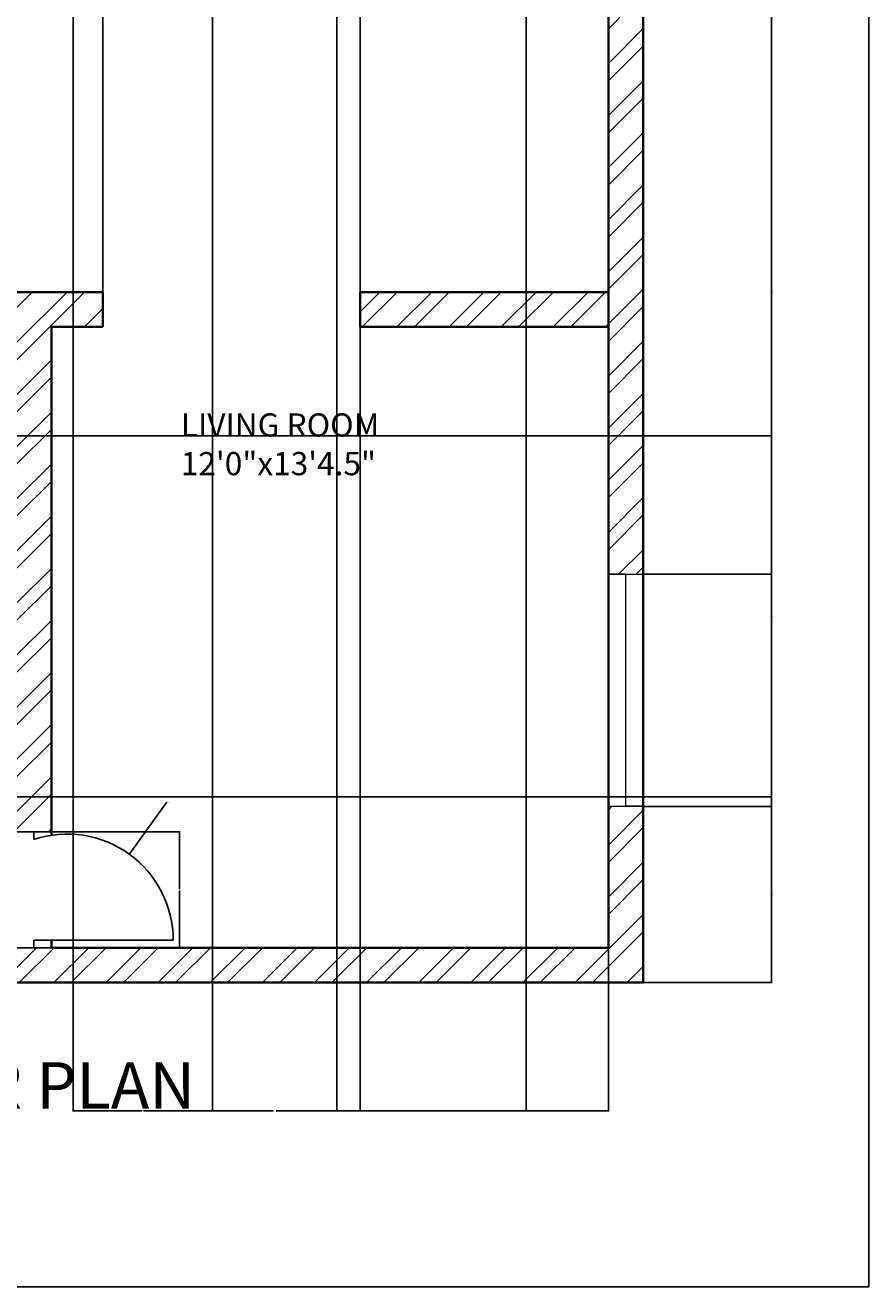
# Model space of a CAD drawing. Units: inches. Extents: x 1595 to 2135, y 460 to 2061.
# Tile 3 of 5: x 1917 to 2135, y 1320 to 1646. Entities that reach past the tile are written whole.
import ezdxf

# ---------------------------------------------------------------- set-up
doc = ezdxf.new("R2010")
doc.units = ezdxf.units.IN
for name, color, linetype, lineweight in [('A-ANNO-DIMS', 2, 'Continuous', 18), ('A-ANNO-TTLB', 7, 'Continuous', 25), ('A-AREA-IDEN', 7, 'Continuous', 18), ('A-DOOR', 3, 'Continuous', 25), ('A-GLAZ', 4, 'Continuous', 18), ('A-WALL', 7, 'Continuous', 35)]:
    doc.layers.add(name, color=color, linetype=linetype, lineweight=lineweight)
doc.layers.add('A-WALL-PATT', color=143, linetype='Continuous', lineweight=13, true_color=0x7aafdf)
doc.styles.get("Standard").update_dxf_attribs({"font": 'arial.ttf'})
doc.dimstyles.get("Standard").update_dxf_attribs({"dimtxt": 0.18, "dimasz": 0.18, "dimexe": 0.18, "dimexo": 0.0625, "dimgap": 0.09, "dimtad": 0, "dimtih": 1, "dimtoh": 1, "dimdec": 4, "dimzin": 0, "dimdsep": 46, "dimtxsty": 'Standard', "dimcen": 0.09, "dimadec": 0, "dimazin": 0, "dimtfac": 1, "dimtdec": 4, "dimtofl": 0, "dimtmove": 0, "dimatfit": 3, "dimfxl": 1, "dimtolj": 1, "dimtzin": 0, "dimarcsym": 0})

# ---------------------------------------------------------------- blocks, each defined once
blk = doc.blocks.new('WIN-60IN')
for p, q in [((4.5, 60), (0, 60)), ((0, 60), (9, 60)), ((4.5, 0), (4.5, 60)), ((0, 0), (9, 0)), ((9, 0), (4.5, 0))]:
    blk.add_line(p, q)
blk = doc.blocks.new('*D14')
at = {"layer": 'A-ANNO-DIMS', "color": 0, "lineweight": -2, "transparency": 16777216}
for p, q in [((2076.38, 1444.2), (2109.64, 1444.2)), ((2109.46, 1444.02), (2109.46, 1421.6)), ((2109.46, 1398.82), (2109.46, 1421.24)), ((2076.38, 1398.64), (2109.64, 1398.64))]:
    blk.add_line(p, q, dxfattribs=at)
at = {"layer": 'A-ANNO-DIMS', "color": 0, "transparency": 16777216}
for points in [[(2109.43, 1444.02), (2109.49, 1444.02), (2109.46, 1444.2)], [(2109.43, 1398.82), (2109.49, 1398.82), (2109.46, 1398.64)]]:
    blk.add_solid(points, dxfattribs=at)
at = {"layer": 'Defpoints', "color": 0, "transparency": 16777216}
for p in [(2076.31, 1444.2), (2109.46, 1444.2), (2076.31, 1398.64)]:
    blk.add_point(p, dxfattribs=at)
at = {"layer": 'A-ANNO-DIMS', "color": 0, "transparency": 16777216, "insert": (2109.46, 1421.42), "char_height": 0.18, "attachment_point": 5}
blk.add_mtext('\\A1;45.56', dxfattribs=at)
blk = doc.blocks.new('*D15')
at = {"layer": 'A-ANNO-DIMS', "color": 0, "lineweight": -2, "transparency": 16777216}
for p, q in [((2076.38, 1650.64), (2109.64, 1650.64)), ((2109.46, 1650.46), (2109.46, 1577.6)), ((2109.46, 1504.38), (2109.46, 1577.24)), ((2076.38, 1504.2), (2109.64, 1504.2))]:
    blk.add_line(p, q, dxfattribs=at)
at = {"layer": 'A-ANNO-DIMS', "color": 0, "transparency": 16777216}
for points in [[(2109.43, 1650.46), (2109.49, 1650.46), (2109.46, 1650.64)], [(2109.43, 1504.38), (2109.49, 1504.38), (2109.46, 1504.2)]]:
    blk.add_solid(points, dxfattribs=at)
at = {"layer": 'Defpoints', "color": 0, "transparency": 16777216}
for p in [(2076.31, 1650.64), (2109.46, 1650.64), (2076.31, 1504.2)]:
    blk.add_point(p, dxfattribs=at)
at = {"layer": 'A-ANNO-DIMS', "color": 0, "transparency": 16777216, "insert": (2109.46, 1577.42), "char_height": 0.18, "attachment_point": 5}
blk.add_mtext('\\A1;146.44', dxfattribs=at)
blk = doc.blocks.new('*D20')
at = {"layer": 'A-ANNO-DIMS', "color": 0, "lineweight": -2, "transparency": 16777216}
for p, q in [((1923.38, 1437.64), (1956.64, 1437.64)), ((1956.46, 1437.46), (1956.46, 1422.82)), ((1956.46, 1407.82), (1956.46, 1422.46)), ((1923.38, 1407.64), (1956.64, 1407.64))]:
    blk.add_line(p, q, dxfattribs=at)
at = {"layer": 'A-ANNO-DIMS', "color": 0, "transparency": 16777216}
for points in [[(1956.43, 1437.46), (1956.49, 1437.46), (1956.46, 1437.64)], [(1956.43, 1407.82), (1956.49, 1407.82), (1956.46, 1407.64)]]:
    blk.add_solid(points, dxfattribs=at)
at = {"layer": 'Defpoints', "color": 0, "transparency": 16777216}
for p in [(1923.31, 1437.64), (1923.31, 1407.64), (1956.46, 1407.64)]:
    blk.add_point(p, dxfattribs=at)
at = {"layer": 'A-ANNO-DIMS', "color": 0, "transparency": 16777216, "insert": (1956.46, 1422.64), "char_height": 0.18, "attachment_point": 5}
blk.add_mtext('\\A1;30', dxfattribs=at)
blk = doc.blocks.new('*D21')
at = {"layer": 'A-ANNO-DIMS', "color": 0, "lineweight": -2, "transparency": 16777216}
for p, q in [((1936.61, 1577.2), (1936.61, 2049.97)), ((1936.79, 2049.79), (1969.47, 2049.79)), ((2002.95, 2049.79), (1970.26, 2049.79)), ((2003.13, 1577.2), (2003.13, 2049.97))]:
    blk.add_line(p, q, dxfattribs=at)
at = {"layer": 'A-ANNO-DIMS', "color": 0, "transparency": 16777216}
for points in [[(1936.79, 2049.82), (1936.79, 2049.76), (1936.61, 2049.79)], [(2002.95, 2049.82), (2002.95, 2049.76), (2003.13, 2049.79)]]:
    blk.add_solid(points, dxfattribs=at)
at = {"layer": 'Defpoints', "color": 0, "transparency": 16777216}
for p in [(2003.13, 2049.79), (1936.61, 1577.14), (2003.13, 1577.14)]:
    blk.add_point(p, dxfattribs=at)
at = {"layer": 'A-ANNO-DIMS', "color": 0, "transparency": 16777216, "insert": (1969.87, 2049.79), "char_height": 0.18, "attachment_point": 5}
blk.add_mtext('\\A1;66.52', dxfattribs=at)
blk = doc.blocks.new('*D22')
at = {"layer": 'A-ANNO-DIMS', "color": 0, "lineweight": -2, "transparency": 16777216}
for p, q in [((2003.13, 1568.08), (2003.13, 1365.31)), ((2067.31, 1568.08), (2067.31, 1365.31)), ((2003.31, 1365.49), (2034.83, 1365.49)), ((2067.13, 1365.49), (2035.62, 1365.49))]:
    blk.add_line(p, q, dxfattribs=at)
at = {"layer": 'A-ANNO-DIMS', "color": 0, "transparency": 16777216}
for points in [[(2003.31, 1365.52), (2003.31, 1365.46), (2003.13, 1365.49)], [(2067.13, 1365.52), (2067.13, 1365.46), (2067.31, 1365.49)]]:
    blk.add_solid(points, dxfattribs=at)
at = {"layer": 'Defpoints', "color": 0, "transparency": 16777216}
for p in [(2003.13, 1568.14), (2067.31, 1568.14), (2067.31, 1365.49)]:
    blk.add_point(p, dxfattribs=at)
at = {"layer": 'A-ANNO-DIMS', "color": 0, "transparency": 16777216, "insert": (2035.22, 1365.49), "char_height": 0.18, "attachment_point": 5}
blk.add_mtext('\\A1;64.18', dxfattribs=at)
blk = doc.blocks.new('*D27')
at = {"layer": 'A-ANNO-DIMS', "color": 0, "lineweight": -2, "transparency": 16777216}
for p, q in [((1997.11, 1938.58), (1997.11, 1365.31)), ((2046.03, 1938.58), (2046.03, 1365.31)), ((1997.29, 1365.49), (2021.18, 1365.49)), ((2045.85, 1365.49), (2021.97, 1365.49))]:
    blk.add_line(p, q, dxfattribs=at)
at = {"layer": 'A-ANNO-DIMS', "color": 0, "transparency": 16777216}
for points in [[(1997.29, 1365.52), (1997.29, 1365.46), (1997.11, 1365.49)], [(2045.85, 1365.52), (2045.85, 1365.46), (2046.03, 1365.49)]]:
    blk.add_solid(points, dxfattribs=at)
at = {"layer": 'Defpoints', "color": 0, "transparency": 16777216}
for p in [(1997.11, 1938.64), (2046.03, 1938.64), (2046.03, 1365.49)]:
    blk.add_point(p, dxfattribs=at)
at = {"layer": 'A-ANNO-DIMS', "color": 0, "transparency": 16777216, "insert": (2021.57, 1365.49), "char_height": 0.18, "attachment_point": 5}
blk.add_mtext('\\A1;48.92', dxfattribs=at)
blk = doc.blocks.new('*D28')
at = {"layer": 'A-ANNO-DIMS', "color": 0, "lineweight": -2, "transparency": 16777216}
for p, q in [((1928.93, 1938.58), (1928.93, 1365.31)), ((1964.93, 1938.58), (1964.93, 1365.31)), ((1929.11, 1365.49), (1946.71, 1365.49)), ((1964.75, 1365.49), (1947.15, 1365.49))]:
    blk.add_line(p, q, dxfattribs=at)
at = {"layer": 'A-ANNO-DIMS', "color": 0, "transparency": 16777216}
for points in [[(1929.11, 1365.52), (1929.11, 1365.46), (1928.93, 1365.49)], [(1964.75, 1365.52), (1964.75, 1365.46), (1964.93, 1365.49)]]:
    blk.add_solid(points, dxfattribs=at)
at = {"layer": 'Defpoints', "color": 0, "transparency": 16777216}
for p in [(1928.93, 1938.64), (1964.93, 1938.64), (1964.93, 1365.49)]:
    blk.add_point(p, dxfattribs=at)
at = {"layer": 'A-ANNO-DIMS', "color": 0, "transparency": 16777216, "insert": (1946.93, 1365.49), "char_height": 0.18, "attachment_point": 5}
blk.add_mtext('\\A1;36', dxfattribs=at)
blk = doc.blocks.new('*D29')
at = {"layer": 'A-ANNO-DIMS', "color": 0, "lineweight": -2, "transparency": 16777216}
for p, q in [((1964.93, 1938.58), (1964.93, 1365.31)), ((1997.11, 1938.58), (1997.11, 1365.31)), ((1965.11, 1365.49), (1980.63, 1365.49)), ((1996.93, 1365.49), (1981.42, 1365.49))]:
    blk.add_line(p, q, dxfattribs=at)
at = {"layer": 'A-ANNO-DIMS', "color": 0, "transparency": 16777216}
for points in [[(1965.11, 1365.52), (1965.11, 1365.46), (1964.93, 1365.49)], [(1996.93, 1365.52), (1996.93, 1365.46), (1997.11, 1365.49)]]:
    blk.add_solid(points, dxfattribs=at)
at = {"layer": 'Defpoints', "color": 0, "transparency": 16777216}
for p in [(1964.93, 1938.64), (1997.11, 1938.64), (1997.11, 1365.49)]:
    blk.add_point(p, dxfattribs=at)
at = {"layer": 'A-ANNO-DIMS', "color": 0, "transparency": 16777216, "insert": (1981.02, 1365.49), "char_height": 0.18, "attachment_point": 5}
blk.add_mtext('\\A1;32.18', dxfattribs=at)
blk = doc.blocks.new('*D34')
at = {"layer": 'A-ANNO-DIMS', "color": 0, "lineweight": -2, "transparency": 16777216}
for p, q in [((1914.38, 1539.98), (2109.64, 1539.98)), ((2109.46, 1539.8), (2109.46, 1493.49)), ((2109.46, 1446.82), (2109.46, 1493.13)), ((1914.38, 1446.64), (2109.64, 1446.64))]:
    blk.add_line(p, q, dxfattribs=at)
at = {"layer": 'A-ANNO-DIMS', "color": 0, "transparency": 16777216}
for points in [[(2109.43, 1539.8), (2109.49, 1539.8), (2109.46, 1539.98)], [(2109.43, 1446.82), (2109.49, 1446.82), (2109.46, 1446.64)]]:
    blk.add_solid(points, dxfattribs=at)
at = {"layer": 'Defpoints', "color": 0, "transparency": 16777216}
for p in [(1914.31, 1539.98), (2109.46, 1539.98), (1914.31, 1446.64)]:
    blk.add_point(p, dxfattribs=at)
at = {"layer": 'A-ANNO-DIMS', "color": 0, "transparency": 16777216, "insert": (2109.46, 1493.31), "char_height": 0.18, "attachment_point": 5}
blk.add_mtext('\\A1;93.33', dxfattribs=at)
blk = doc.blocks.new('*D46')
at = {"layer": 'A-ANNO-DIMS', "color": 0, "lineweight": -2, "transparency": 16777216}
for p, q in [((2076.38, 2016.64), (2109.64, 2016.64)), ((2109.46, 2016.46), (2109.46, 1707.82)), ((2109.46, 1398.82), (2109.46, 1707.46)), ((2076.38, 1398.64), (2109.64, 1398.64))]:
    blk.add_line(p, q, dxfattribs=at)
at = {"layer": 'A-ANNO-DIMS', "color": 0, "transparency": 16777216}
for points in [[(2109.43, 2016.46), (2109.49, 2016.46), (2109.46, 2016.64)], [(2109.43, 1398.82), (2109.49, 1398.82), (2109.46, 1398.64)]]:
    blk.add_solid(points, dxfattribs=at)
at = {"layer": 'Defpoints', "color": 0, "transparency": 16777216}
for p in [(2076.31, 2016.64), (2109.46, 2016.64), (2076.31, 1398.64)]:
    blk.add_point(p, dxfattribs=at)
at = {"layer": 'A-ANNO-DIMS', "color": 0, "transparency": 16777216, "insert": (2109.46, 1707.64), "char_height": 0.18, "attachment_point": 5}
blk.add_mtext('\\A1;618', dxfattribs=at)
blk = doc.blocks.new('*D59')
at = {"layer": 'A-ANNO-DIMS', "color": 0, "lineweight": -2, "transparency": 16777216}
for p, q in [((1953.08, 1445.17), (1943.57, 1431.99)), ((1953.26, 1445.17), (1953.08, 1445.17)), ((1927.33, 1409.64), (1927.51, 1409.64)), ((1927.42, 1409.55), (1927.42, 1409.73))]:
    blk.add_line(p, q, dxfattribs=at)
at = {"layer": 'A-ANNO-DIMS', "color": 0, "transparency": 16777216}
blk.add_solid([(1943.54, 1432.01), (1943.59, 1431.97), (1943.46, 1431.85)], dxfattribs=at)
at = {"layer": 'Defpoints', "color": 0, "transparency": 16777216}
for p in [(1943.46, 1431.85), (1927.42, 1409.64)]:
    blk.add_point(p, dxfattribs=at)
at = {"layer": 'A-ANNO-DIMS', "color": 0, "transparency": 16777216, "insert": (1953.74, 1445.17), "char_height": 0.18, "attachment_point": 5}
blk.add_mtext('\\A1;R27.39', dxfattribs=at)

msp = doc.modelspace()

# ---------------------------------------------------------------- hatches: boundary and pattern name
at = {"layer": 'A-WALL-PATT'}
h = msp.add_hatch(dxfattribs=at)
h.set_pattern_fill('ANSI32', color=256)
h.paths.add_polyline_path([(2076.313, 2016.6421), (1674.313, 2016.6421), (1674.313, 1905.0731), (1683.313, 1905.0731), (1683.313, 1938.6421), (1705.9756, 1938.6421), (1705.9756, 1947.6421), (1683.313, 1947.6421), (1683.313, 2007.6421), (2067.313, 2007.6421), (2067.313, 1947.6421), (2046.0304, 1947.6421), (2046.0304, 1938.6421), (2067.313, 1938.6421), (2067.313, 1906.0373), (2076.313, 1906.0373), (2076.313, 1947.6421)])
h.paths.add_polyline_path([(1786.653, 1947.6421), (1748.8699, 1947.6421), (1748.8699, 1938.6421), (1786.653, 1938.6421), (1786.653, 1943.1421)], flags=17)
h.paths.add_polyline_path([(1843.367, 1943.1421), (1843.367, 1947.6421), (1822.653, 1947.6421), (1822.653, 1938.6421), (1827.313, 1938.6421), (1827.313, 1821.1082), (1836.313, 1821.1082), (1836.313, 1938.6421), (1843.367, 1938.6421)])
h.paths.add_polyline_path([(1928.933, 1943.1421), (1928.933, 1947.6421), (1875.313, 1947.6421), (1875.313, 1938.6421), (1914.313, 1938.6421), (1914.313, 1820.8892), (1923.313, 1820.8892), (1923.313, 1938.6421), (1928.933, 1938.6421)])
h.paths.add_polyline_path([(1997.1133, 1947.6421), (1964.933, 1947.6421), (1964.933, 1938.6421), (1997.1133, 1938.6421)], flags=17)
h.paths.add_polyline_path([(1974.313, 2007.6421), (1969.813, 2007.6421), (1969.813, 1947.6421), (1974.313, 1947.6421)], flags=17)
h.paths.add_polyline_path([(1780.813, 2007.6421), (1776.313, 2007.6421), (1776.313, 1947.6421), (1780.813, 1947.6421)], flags=17)
h.paths.add_polyline_path([(1683.313, 1845.0731), (1674.313, 1845.0731), (1674.313, 1734.209), (1683.313, 1734.209), (1683.313, 1773.6421), (1795.813, 1773.6421), (1836.313, 1773.6421), (1836.313, 1788.3627), (1831.813, 1788.3627), (1827.313, 1788.3627), (1827.313, 1782.6421), (1683.313, 1782.6421)])
h.paths.add_polyline_path([(2076.313, 1846.0373), (2067.313, 1846.0373), (2067.313, 1782.6421), (1923.313, 1782.6421), (1923.313, 1788.8802), (1918.813, 1788.8802), (1914.313, 1788.8802), (1914.313, 1773.6421), (2067.313, 1773.6421), (2067.313, 1710.6421), (2076.313, 1710.6421)])
h.paths.add_polyline_path([(1844.0531, 1859.9747), (1909.4596, 1859.9747), (1909.4596, 1882.3635), (1844.0531, 1882.3635)], flags=9)
h.paths.add_polyline_path([(1721.6058, 1827.3507), (1768.2143, 1827.3507), (1768.2143, 1849.7395), (1721.6058, 1849.7395)], flags=9)
h.paths.add_polyline_path([(1786.8661, 1359.2872), (1978.2276, 1359.2872), (1978.2276, 1384.0157), (1786.8661, 1384.0157)], flags=9)
h.paths.add_polyline_path([(1795.7228, 1412.0413), (1871.5904, 1412.0413), (1871.5904, 1424.4055), (1795.7228, 1424.4055)], flags=9)
h.paths.add_polyline_path([(1954.3634, 1526.3976), (2013.549, 1526.3976), (2013.549, 1548.7864), (1954.3634, 1548.7864)], flags=9)
h.paths.add_polyline_path([(1871.0596, 1490.4707), (1913.1292, 1490.4707), (1913.1292, 1512.8595), (1871.0596, 1512.8595)], flags=9)
h.paths.add_polyline_path([(1810.9452, 1510.8402), (1845.9343, 1510.8402), (1845.9343, 1533.229), (1810.9452, 1533.229)], flags=9)
h.paths.add_polyline_path([(1720.9117, 1692.9695), (1767.819, 1692.9695), (1767.819, 1715.3583), (1720.9117, 1715.3583)], flags=9)
h.paths.add_polyline_path([(1853.0254, 1698.4614), (1904.6966, 1698.4614), (1904.6966, 1720.8503), (1853.0254, 1720.8503)], flags=9)
h.paths.add_polyline_path([(1970.399, 1827.3507), (2017.0075, 1827.3507), (2017.0075, 1849.7395), (1970.399, 1849.7395)], flags=9)
h.paths.add_polyline_path([(1994.3418, 1955.5613), (2029.5928, 1955.5613), (2029.5928, 1977.9501), (1994.3418, 1977.9501)], flags=25)
h.paths.add_polyline_path([(1828.8665, 1964.6116), (1868.5173, 1964.6116), (1868.5173, 1987.0004), (1828.8665, 1987.0004)], flags=25)
h.paths.add_polyline_path([(1698.1483, 1960.8371), (1733.3994, 1960.8371), (1733.3994, 1983.2259), (1698.1483, 1983.2259)], flags=25)
h = msp.add_hatch(dxfattribs=at)
h.set_pattern_fill('ANSI32', color=256)
h.paths.add_polyline_path([(1683.313, 1641.6421), (1791.313, 1641.6421), (1791.313, 1634.7169), (1800.313, 1634.7169), (1800.313, 1650.6421), (1800.313, 1673.3054), (1795.813, 1673.3054), (1795.813, 1650.6421), (1683.313, 1650.6421), (1683.313, 1698.209), (1678.813, 1698.209), (1674.313, 1698.209), (1674.313, 1398.6421), (1688.853, 1398.6421), (1688.853, 1403.1421), (1688.853, 1407.6421), (1683.313, 1407.6421)])
h.paths.add_polyline_path([(1800.313, 1568.1421), (1827.2399, 1568.1421), (1827.2399, 1572.6421), (1827.2399, 1577.1421), (1800.313, 1577.1421), (1800.313, 1604.9472), (1795.813, 1604.9472), (1791.313, 1604.9472), (1791.313, 1437.6421), (1800.313, 1437.6421), (1815.6708, 1437.6421), (1815.6708, 1442.1421), (1815.6708, 1446.6421), (1800.313, 1446.6421)])
h.paths.add_polyline_path([(1877.5816, 1545.4284), (1877.5816, 1548.9761), (1864.813, 1548.9761), (1864.813, 1577.1421), (1852.144, 1577.1421), (1852.144, 1568.1421), (1860.313, 1568.1421), (1860.313, 1446.6421), (1839.6708, 1446.6421), (1839.6708, 1437.6421), (1869.0647, 1437.6421), (1869.0647, 1442.1421), (1869.0647, 1446.6421), (1864.813, 1446.6421), (1864.813, 1539.9761), (1877.5816, 1539.9761), (1877.5816, 1541.8808)])
h.paths.add_polyline_path([(1923.313, 1568.1421), (1936.607, 1568.1421), (1936.607, 1577.1421), (1914.313, 1577.1421), (1914.313, 1548.9761), (1901.5816, 1548.9761), (1901.5816, 1539.9761), (1914.313, 1539.9761), (1914.313, 1446.6421), (1891.5684, 1446.6421), (1891.5684, 1437.6421), (1914.313, 1437.6421), (1923.313, 1437.6421)])
h.paths.add_polyline_path([(2067.313, 1577.1421), (2003.1294, 1577.1421), (2003.1294, 1568.1421), (2067.313, 1568.1421)])
h.paths.add_polyline_path([(2076.313, 1650.6421), (2067.313, 1650.6421), (2067.313, 1504.2035), (2076.313, 1504.2035)])
h.paths.add_polyline_path([(2076.313, 1444.2035), (2071.813, 1444.2035), (2067.313, 1444.2035), (2067.313, 1407.6421), (1923.313, 1407.6421), (1918.813, 1407.6421), (1914.313, 1407.6421), (1737.2767, 1407.6421), (1737.2767, 1398.6421), (2076.313, 1398.6421)])

# ---------------------------------------------------------------- linework, layer by layer
at = {"layer": 'A-ANNO-TTLB'}
msp.add_lwpolyline([(1595.2754, 2061.0707), (2134.6206, 2061.0707), (2134.6206, 1319.9937), (1595.2754, 1319.9937)], close=True, dxfattribs=at)
at = {"layer": 'A-DOOR'}
for p, q in [((1914.313, 1437.6421), (1923.313, 1437.6421)), ((1923.313, 1437.6421), (1918.813, 1437.6421)), ((1918.813, 1437.6421), (1918.813, 1435.6421)), ((1918.813, 1407.6421), (1918.813, 1409.6421)), ((1918.813, 1409.6421), (1954.813, 1409.6421)), ((1914.313, 1407.6421), (1923.313, 1407.6421)), ((1923.313, 1407.6421), (1918.813, 1407.6421))]:
    msp.add_line(p, q, dxfattribs=at)
msp.add_arc((1927.4241, 1409.6421), 27.3889, 360, 108.324694, dxfattribs=at)
at = {"layer": 'A-WALL'}
for p, q in [((2076.313, 1947.6421), (2076.313, 1398.6421)), ((2067.313, 1407.6421), (2067.313, 1650.6421)), ((1914.313, 1577.1421), (1936.607, 1577.1421)), ((1936.607, 1577.1421), (1936.607, 1568.1421)), ((2003.1294, 1577.1421), (2003.1294, 1568.1421)), ((2003.1294, 1577.1421), (2067.313, 1577.1421)), ((1923.313, 1568.1421), (1936.607, 1568.1421)), ((1923.313, 1436.7206), (1923.313, 1568.1421)), ((2003.1294, 1568.1421), (2067.313, 1568.1421)), ((1923.313, 1407.6421), (1923.313, 1409.6421)), ((2067.313, 1407.6421), (1923.313, 1407.6421)), ((1923.313, 1407.6421), (2067.313, 1407.6421)), ((1737.2767, 1398.6421), (2076.313, 1398.6421))]:
    msp.add_line(p, q, dxfattribs=at)

# ---------------------------------------------------------------- block references
at = {"layer": 'A-GLAZ'}
msp.add_blockref('WIN-60IN', (2067.313, 1444.203), dxfattribs=at)

# ---------------------------------------------------------------- texts
at = {"layer": 'A-ANNO-TTLB', "insert": (1790.7583, 1378.0525), "char_height": 12, "attachment_point": 1, "line_spacing_factor": 2.88}
msp.add_mtext_dynamic_manual_height_columns('GROUND FLOOR PLAN ', width=392.566159, gutter_width=12.5, heights=[0], dxfattribs=at)
at = {"layer": 'A-AREA-IDEN', "insert": (1956.7761, 1545.8048), "char_height": 6, "attachment_point": 1}
msp.add_mtext_dynamic_manual_height_columns('LIVING ROOM\\P12\'0"x13\'4.5"', width=171.27339, gutter_width=12.5, heights=[0], dxfattribs=at)

# ---------------------------------------------------------------- dimensions: what is measured, and where the dimension line sits
at = {"layer": 'A-ANNO-DIMS'}
for base, p1, p2, override, picture, middle in [((2003.1294, 2049.7921), (1936.607, 1577.1421), (2003.1294, 1577.1421), {"dimdec": 2, "dimlfac": 1, "dimrnd": 0, "dimzin": 0, "dimdsep": 46, "dimlunit": 2}, '*D21', (1969.8682, 2049.7921)), ((1964.933, 1365.4921), (1928.933, 1938.6421), (1964.933, 1938.6421), {"dimdec": 0, "dimlfac": 1, "dimrnd": 0, "dimzin": 0, "dimdsep": 46, "dimlunit": 2}, '*D28', (1946.933, 1365.4921)), ((1997.1133, 1365.4921), (1964.933, 1938.6421), (1997.1133, 1938.6421), {"dimdec": 2, "dimlfac": 1, "dimrnd": 0, "dimzin": 0, "dimdsep": 46, "dimlunit": 2}, '*D29', (1981.0231, 1365.4921)), ((2046.0304, 1365.4921), (1997.1133, 1938.6421), (2046.0304, 1938.6421), {"dimdec": 2, "dimlfac": 1, "dimrnd": 0, "dimzin": 0, "dimdsep": 46, "dimlunit": 2}, '*D27', (2021.5719, 1365.4921)), ((2067.313, 1365.4921), (2003.1294, 1568.1421), (2067.313, 1568.1421), {"dimdec": 2, "dimlfac": 1, "dimrnd": 0, "dimzin": 0, "dimdsep": 46, "dimlunit": 2}, '*D22', (2035.2212, 1365.4921))]:
    dim = msp.add_linear_dim(base=base, p1=p1, p2=p2, dimstyle='Standard', override=override, dxfattribs=at)
    dim.commit()
    dim.dimension.update_dxf_attribs({"geometry": picture, "text_midpoint": middle})
for base, p1, p2, angle, override, picture, middle in [((2109.463, 2016.6421), (2076.313, 1398.6421), (2076.313, 2016.6421), 90, {"dimdec": 0, "dimlfac": 1, "dimrnd": 0, "dimzin": 0, "dimdsep": 46, "dimlunit": 2}, '*D46', (2109.463, 1707.6421)), ((2109.463, 1650.6421), (2076.313, 1504.2035), (2076.313, 1650.6421), 90, {"dimdec": 2, "dimlfac": 1, "dimrnd": 0, "dimzin": 0, "dimdsep": 46, "dimlunit": 2}, '*D15', (2109.463, 1577.4228)), ((2109.463, 1539.9761), (1914.313, 1446.6421), (1914.313, 1539.9761), 90, {"dimdec": 2, "dimlfac": 1, "dimrnd": 0, "dimzin": 0, "dimdsep": 46, "dimlunit": 2}, '*D34', (2109.463, 1493.3091)), ((2109.463, 1444.2035), (2076.313, 1398.6421), (2076.313, 1444.2035), 90, {"dimdec": 2, "dimlfac": 1, "dimrnd": 0, "dimzin": 0, "dimdsep": 46, "dimlunit": 2}, '*D14', (2109.463, 1421.4228)), ((1956.463, 1407.6421), (1923.313, 1437.6421), (1923.313, 1407.6421), 270, {"dimdec": 0, "dimlfac": 1, "dimrnd": 0, "dimzin": 0, "dimdsep": 46, "dimlunit": 2}, '*D20', (1956.463, 1422.6421))]:
    dim = msp.add_linear_dim(base=base, p1=p1, p2=p2, angle=angle, dimstyle='Standard', override=override, dxfattribs=at)
    dim.commit()
    dim.dimension.update_dxf_attribs({"geometry": picture, "text_midpoint": middle})
dim = msp.add_radius_dim(center=(1927.4241, 1409.6421), mpoint=(1943.4599, 1431.8458), dimstyle='Standard', override={"dimdec": 2, "dimlfac": 1, "dimrnd": 0, "dimzin": 0, "dimdsep": 46, "dimlunit": 2}, dxfattribs=at)
dim.commit()
dim.dimension.update_dxf_attribs({"geometry": '*D59', "text_midpoint": (1953.7413, 1445.1681), "dimtype": 164})

doc.saveas('drawing.dxf')
